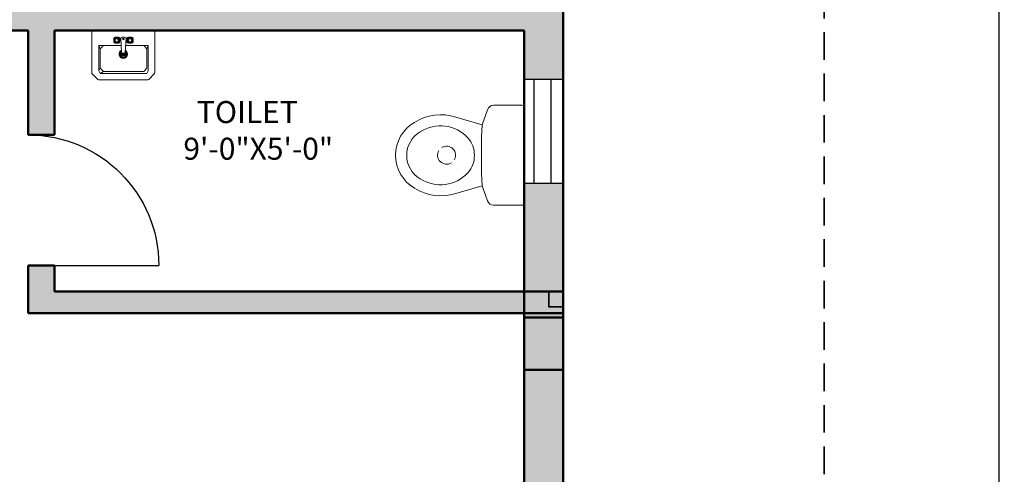
# Model space of a CAD drawing. Units: inches. Extents: x -7 to 1228, y -146 to 1091.
# Tile 41 of 88: x 1002 to 1228, y 200 to 304. Entities that reach past the tile are written whole.
import ezdxf

# ---------------------------------------------------------------- set-up
doc = ezdxf.new("R2010")
doc.units = ezdxf.units.IN
doc.linetypes.add('DASHED2', pattern=[9.525, 6.35, -3.175])
for name, color, linetype, lineweight in [('A-ANNO-DIMS', 2, 'Continuous', 18), ('A-AREA-IDEN', 7, 'Continuous', 18), ('A-COLS', 6, 'Continuous', 35), ('A-DOOR', 4, 'Continuous', 25), ('A-FLOR-FIXT', 8, 'Continuous', 18), ('A-FURN', 8, 'Continuous', 18), ('A-GLAZ', 175, 'Continuous', 25), ('A-WALL', 7, 'Continuous', 50), ('A-WALL-PATT', 251, 'Continuous', 13), ('C-PROP', 1, 'DASHED2', 35)]:
    doc.layers.add(name, color=color, linetype=linetype, lineweight=lineweight)
doc.styles.get("Standard").update_dxf_attribs({"font": 'arial.ttf'})
doc.dimstyles.new('ISO-25', dxfattribs={"dimtxt": 7, "dimasz": 4, "dimexe": 1.25, "dimexo": 0.625, "dimtad": 1, "dimdec": 1, "dimlunit": 3, "dimtxsty": 'Standard', "dimcen": 2.5, "dimadec": 0, "dimazin": 0, "dimtfac": 1, "dimtdec": 1, "dimtmove": 1, "dimatfit": 3, "dimfxl": 1, "dimarcsym": 0})

# ---------------------------------------------------------------- blocks, each defined once
blk = doc.blocks.new('A$C7B5C7CD4')
at = {"ltscale": 20}
for p, q in [((0.243, 0.625), (0.011, 0.625)), ((0.243, 0.625), (0.475, 0.625)), ((0, 0.614), (0, 0.4765)), ((0.486, 0.614), (0.486, 0.4765)), ((0.0212, 0.4467), (0.0946, 0.4214)), ((0.4648, 0.4467), (0.3914, 0.4214)), ((0.0946, 0.4214), (0.0576, 0.293)), ((0.0946, 0.4214), (0.1544, 0.4173)), ((0.3316, 0.4173), (0.1544, 0.4173)), ((0.3914, 0.4214), (0.3316, 0.4173)), ((0.3914, 0.4214), (0.4284, 0.293))]:
    blk.add_line(p, q, dxfattribs=at)
for centre, radius, start, end in [((0.011, 0.614), 0.011, 90, 180), ((0.475, 0.614), 0.011, 0, 90), ((0.0315, 0.4765), 0.0315, 180, 251), ((0.4545, 0.4765), 0.0315, 289, 0), ((0.2796, 0.219), 0.18, 132.4207, 213.289), ((0.24, 0.2602), 0.123, 88.6158, 131.7414), ((0.246, 0.2602), 0.123, 48.2586, 91.3842), ((0.2064, 0.219), 0.18, 326.711, 47.5793), ((0.2796, 0.219), 0.234, 161.5846, 212.8753), ((0.2064, 0.219), 0.234, 327.1247, 18.4154), ((0.243, 0.185), 0.131, 209.6292, 270), ((0.243, 0.185), 0.131, 270, 330.3708), ((0.243, 0.185), 0.185, 210.1745, 270), ((0.243, 0.185), 0.185, 270, 329.8255)]:
    blk.add_arc(centre, radius, start, end, dxfattribs=at)
for start, end in [(58.1785, 211.8215), (238.1785, 31.8215)]:
    blk.add_arc((0.2426, 0.2481), 0.0439, start, end)
blk = doc.blocks.new('*D12')
at = {"layer": 'A-ANNO-DIMS', "color": 0, "lineweight": -2, "transparency": 16777216}
for p, q in [((1187.62, 1061), (1228.45, 1061)), ((1227.2, 1057), (1227.2, 4)), ((1187.62, 0), (1228.45, 0))]:
    blk.add_line(p, q, dxfattribs=at)
at = {"layer": 'A-ANNO-DIMS', "color": 0, "transparency": 16777216}
for points in [[(1226.53, 1057), (1227.86, 1057), (1227.2, 1061)], [(1226.53, 4), (1227.86, 4), (1227.2, 0)]]:
    blk.add_solid(points, dxfattribs=at)
at = {"layer": 'Defpoints', "color": 0, "transparency": 16777216}
for p in [(1187, 1061), (1187, 0), (1227.2, 0)]:
    blk.add_point(p, dxfattribs=at)
at = {"layer": 'A-ANNO-DIMS', "color": 0, "transparency": 16777216, "insert": (1223, 530.5), "char_height": 7, "attachment_point": 5, "rotation": 90}
blk.add_mtext('88\'-5"', dxfattribs=at)
blk = doc.blocks.new('A$C4CB854FF')
for p, q in [((0.4725, 0.38), (0.0125, 0.38)), ((0, 0.3675), (0, 0.0552)), ((0.1677, 0.2932), (0.1677, 0.318)), ((0.1745, 0.2919), (0.1745, 0.3194)), ((0.1773, 0.3221), (0.2048, 0.3221)), ((0.1787, 0.329), (0.2034, 0.329)), ((0.2075, 0.3194), (0.2075, 0.2919)), ((0.2144, 0.318), (0.2144, 0.2932)), ((0.2279, 0.2104), (0.2213, 0.3235)), ((0.2337, 0.329), (0.2502, 0.329)), ((0.2625, 0.3235), (0.256, 0.2104)), ((0.2694, 0.318), (0.2694, 0.2932)), ((0.2763, 0.3194), (0.2763, 0.2919)), ((0.3065, 0.3221), (0.279, 0.3221)), ((0.3052, 0.329), (0.2804, 0.329)), ((0.3093, 0.2919), (0.3093, 0.3194)), ((0.3162, 0.2932), (0.3162, 0.318)), ((0.485, 0.0552), (0.485, 0.3675)), ((0.05, 0.265), (0.2247, 0.265)), ((0.06, 0.24), (0.05, 0.265)), ((0.05, 0.07), (0.05, 0.265)), ((0.085, 0.265), (0.06, 0.24)), ((0.06, 0.24), (0.06, 0.09)), ((0.2048, 0.2891), (0.1773, 0.2891)), ((0.2034, 0.2822), (0.1787, 0.2822)), ((0.2591, 0.265), (0.43, 0.265)), ((0.279, 0.2891), (0.3065, 0.2891)), ((0.2804, 0.2822), (0.3052, 0.2822)), ((0.395, 0.265), (0.42, 0.24)), ((0.42, 0.24), (0.43, 0.265)), ((0.42, 0.24), (0.42, 0.09)), ((0.43, 0.07), (0.43, 0.265)), ((0.2152, 0.1984), (0.2694, 0.1984)), ((0.2297, 0.2066), (0.2165, 0.2066)), ((0.2681, 0.1901), (0.2165, 0.1901)), ((0.2272, 0.2149), (0.2208, 0.2149)), ((0.2638, 0.1819), (0.2208, 0.1819)), ((0.2533, 0.1736), (0.2313, 0.1736)), ((0.2505, 0.2052), (0.2334, 0.2052)), ((0.2681, 0.2066), (0.2541, 0.2066)), ((0.2638, 0.2149), (0.2566, 0.2149)), ((0.06, 0.09), (0.085, 0.065)), ((0.42, 0.09), (0.395, 0.065)), ((0.42, 0.09), (0.43, 0.07)), ((0.0037, 0.0463), (0.0463, 0.0037)), ((0.05, 0.07), (0.06, 0.05)), ((0.42, 0.05), (0.06, 0.05)), ((0.085, 0.065), (0.395, 0.065)), ((0.395, 0.065), (0.42, 0.05)), ((0.43, 0.07), (0.42, 0.05)), ((0.4387, 0.0037), (0.4813, 0.0463)), ((0.0552, 0), (0.4298, 0))]:
    blk.add_line(p, q)
for centre, radius in [((0.191, 0.3056), 0.0165), ((0.191, 0.3056), 0.0127), ((0.2419, 0.3152), 0.00688), ((0.2419, 0.3152), 0.00344), ((0.2928, 0.3056), 0.0165), ((0.2928, 0.3056), 0.0127)]:
    blk.add_circle(centre, radius)
for centre, radius, start, end in [((0.0125, 0.3675), 0.0125, 90, 180), ((0.4725, 0.3675), 0.0125, 0, 90), ((0.1787, 0.318), 0.011, 90, 180), ((0.1773, 0.3194), 0.00275, 90, 180), ((0.2034, 0.318), 0.011, 0, 90), ((0.2048, 0.3194), 0.00275, 360, 90), ((0.2329, 0.314), 0.015, 87.19754, 140.72744), ((0.2509, 0.314), 0.015, 39.27256, 92.80246), ((0.2804, 0.318), 0.011, 90, 180), ((0.279, 0.3194), 0.00275, 90, 180), ((0.3052, 0.318), 0.011, 0, 90), ((0.3065, 0.3194), 0.00275, 360, 90), ((0.1787, 0.2932), 0.011, 180, 270), ((0.1773, 0.2919), 0.00275, 180, 270), ((0.2034, 0.2932), 0.011, 270, 0), ((0.2048, 0.2919), 0.00275, 270, 0), ((0.2423, 0.1984), 0.033, 118.68833, 62.86857), ((0.2804, 0.2932), 0.011, 180, 270), ((0.279, 0.2919), 0.00275, 180, 270), ((0.3052, 0.2932), 0.011, 270, 360), ((0.3065, 0.2919), 0.00275, 270, 0), ((0.2423, 0.1984), 0.0271, 124.77581, 57.22467), ((0.2334, 0.2107), 0.0055, 183.3274, 270), ((0.2505, 0.2107), 0.0055, 270, 356.6726), ((0.0125, 0.0552), 0.0125, 180, 225), ((0.0552, 0.0125), 0.0125, 225, 270), ((0.4298, 0.0125), 0.0125, 270, 315), ((0.4725, 0.0552), 0.0125, 315, 0)]:
    blk.add_arc(centre, radius, start, end)
blk = doc.blocks.new('WIN-24')
for p, q in [((0, 0), (0, 24)), ((0, 24), (9, 24)), ((2.34, 0), (2.34, 24)), ((2.34, 24), (6.14, 24)), ((6.14, 24), (6.14, 0)), ((9, 24), (9, 0)), ((9, 0), (0, 0))]:
    blk.add_line(p, q)
blk = doc.blocks.new('DOOR-750')
blk.add_line((30, 30), (30, 0))
blk.add_arc((30, 30), 30, 180, 270)

msp = doc.modelspace()

# ---------------------------------------------------------------- hatches: boundary and pattern name
at = {"layer": 'A-COLS'}
h = msp.add_hatch(color=256, dxfattribs=at)
h.dxf.hatch_style = 1
h.paths.add_polyline_path([(1127, 238.45), (1123.71, 238.45), (1123.71, 242), (1118, 242), (1118, 224), (1127, 224)])
h = msp.add_hatch(color=256, dxfattribs=at)
h.dxf.hatch_style = 1
h.paths.add_polyline_path([(1127, 238.45), (1127, 242), (1123.71, 242), (1123.71, 238.45)])
at = {"layer": 'A-WALL-PATT'}
h = msp.add_hatch(color=256, dxfattribs=at)
h.dxf.hatch_style = 1
h.paths.add_polyline_path([(69, 568), (60, 568), (60, 493), (63.29, 493), (69, 493)])
h.paths.add_polyline_path([(69, 662.41), (60, 662.41), (60, 586), (69, 586)], flags=17)
h.paths.add_polyline_path([(69, 723), (184, 723), (184, 734), (179, 734), (179, 728), (69, 728), (69, 741.62), (60, 741.62), (60, 698.41), (69, 698.41)], flags=17)
h.paths.add_polyline_path([(69, 782), (231, 782), (231, 728), (231, 723), (231, 586), (236, 586), (236, 787), (69, 787), (69, 800.13), (60, 800.13), (60, 765.62), (69, 765.62)])
h.paths.add_polyline_path([(184, 842), (189, 842), (189, 848), (173, 848), (173, 842), (179, 842), (179, 787), (184, 787)])
h.paths.add_polyline_path([(118.22, 69), (69, 69), (69, 60), (118.22, 60)])
h.paths.add_polyline_path([(227, 69), (154.22, 69), (154.22, 60), (227, 60)])
h.paths.add_polyline_path([(236, 60), (232.71, 60), (227, 60), (227, 36), (236, 36)])
h.paths.add_polyline_path([(389, 60), (380, 60), (380, 36), (389, 36)])
h.paths.add_polyline_path([(384, 181), (380, 181), (380, 115), (380, 78), (384, 78)])
h.paths.add_polyline_path([(380, 115), (334.55, 115), (334.55, 109), (380, 109)])
h.paths.add_polyline_path([(274.55, 115), (236, 115), (236, 201), (232.71, 201), (231, 201), (231, 78), (236, 78), (236, 109), (274.55, 109)])
h.paths.add_polyline_path([(69, 123), (60, 123), (60, 78), (69, 78)])
h.paths.add_polyline_path([(69, 201), (60, 201), (60, 159), (69, 159)])
h.paths.add_polyline_path([(143, 219), (69, 219), (69, 213), (143, 213)], flags=17)
h.paths.add_polyline_path([(189, 219), (184, 219), (184, 274), (231, 274), (231, 219), (236, 219), (236, 279), (184, 279), (184, 297), (179, 297), (179, 279), (69, 279), (69, 290.91), (60, 290.91), (60, 262.18), (69, 262.18), (69, 274), (179, 274), (179, 219), (173, 219), (173, 213), (189, 213)])
h.paths.add_polyline_path([(69, 238.18), (60, 238.18), (60, 219), (69, 219)], flags=17)
h.paths.add_polyline_path([(69, 333), (60, 333), (60, 314.91), (69, 314.91), (69, 316.96)])
h.paths.add_polyline_path([(190, 338), (184, 338), (69, 338), (69, 333), (179, 333), (179, 327), (184, 327), (184, 333.02), (190, 333.05)])
h.paths.add_polyline_path([(69, 386.81), (60, 386.81), (60, 351), (69, 351)])
h.paths.add_polyline_path([(69, 475), (60, 475), (60, 422.81), (69, 422.81)])
h.paths.add_polyline_path([(236, 475), (231, 475), (231, 351.24), (236, 351.24)])
h.paths.add_polyline_path([(384, 475), (380, 475), (380, 362), (384, 362)])
h.paths.add_polyline_path([(547, 307), (439, 307), (439, 356), (445, 356), (445, 362), (433, 362), (433, 307), (380, 307), (380, 244), (380, 241), (384, 241), (384, 301), (433, 301), (433, 277), (439, 277), (439, 301), (547, 301)])
h.paths.add_polyline_path([(547, 241), (439, 241), (439, 247), (433, 247), (433, 235), (547, 235)])
h.paths.add_polyline_path([(450, 69), (440.29, 69), (424.89, 69), (389, 69), (389, 60), (450, 60)])
h.paths.add_polyline_path([(547, 69), (486, 69), (486, 60), (547, 60)])
h.paths.add_polyline_path([(556, 148.27), (547, 148.27), (547, 78), (556, 78)])
h.paths.add_polyline_path([(556, 223), (547, 223), (547, 195), (547, 184.27), (556, 184.27)])
h.paths.add_polyline_path([(556, 311.19), (547, 311.19), (547, 273.08), (556, 273.08)])
h.paths.add_polyline_path([(556, 344), (552.71, 344), (547, 344), (547, 335.19), (556, 335.19)])
h.paths.add_polyline_path([(556, 249.08), (547, 249.08), (547, 241), (556, 241)])
h.paths.add_polyline_path([(547, 362), (475, 362), (475, 356), (547, 356)], flags=0)
h.paths.add_polyline_path([(556, 399.62), (547, 399.62), (547, 362), (556, 362)])
h.paths.add_polyline_path([(556, 475), (547, 475), (547, 435.62), (556, 435.62)])
h.paths.add_polyline_path([(547, 493), (389, 493), (389, 487), (547, 487)])
h.paths.add_polyline_path([(380, 493), (278, 493), (278, 487), (380, 487)])
h.paths.add_polyline_path([(227, 493), (69, 493), (69, 487), (227, 487)])
h.paths.add_polyline_path([(643, 122.44), (634, 122.44), (634, 78), (643, 78)])
h.paths.add_polyline_path([(702.5, 69), (692.79, 69), (677.39, 69), (643, 69), (643, 60), (702.5, 60)])
h.paths.add_polyline_path([(798, 69), (738.5, 69), (738.5, 60), (798, 60)])
h.paths.add_polyline_path([(807, 60), (803.71, 60), (798, 60), (798, 36), (807, 36)])
h.paths.add_polyline_path([(807, 109), (846.75, 109), (846.75, 115), (807, 115), (807, 159), (802, 159), (802, 78), (807, 78)])
h.paths.add_polyline_path([(807, 201), (802, 201), (802, 195), (807, 195)])
h.paths.add_polyline_path([(643, 201), (634, 201), (634, 158.44), (643, 158.44)])
h.paths.add_polyline_path([(756, 225), (751, 225), (751, 219), (643, 219), (643, 213), (756, 213)])
h.paths.add_polyline_path([(643, 240.85), (634, 240.85), (634, 219), (643, 219)])
h.paths.add_polyline_path([(643, 274), (643, 288.63), (634, 288.63), (634, 264.85), (643, 264.85)])
h.paths.add_polyline_path([(802, 279), (756, 279), (756, 297), (751, 297), (751, 279), (643, 279), (643, 274), (751, 274), (751, 255), (756, 255), (756, 274), (802, 274)])
h.paths.add_polyline_path([(807, 333), (803.71, 333), (802, 333), (802, 279), (802, 274), (802, 219), (807, 219)])
h.paths.add_polyline_path([(956, 182), (951, 182), (951, 115), (906.75, 115), (906.75, 109), (951, 109), (951, 78), (956, 78)])
h.paths.add_polyline_path([(960, 60), (951, 60), (951, 36), (960, 36)])
h.paths.add_polyline_path([(1021, 69), (1005.78, 69), (960, 69), (960, 60), (1021, 60)])
h.paths.add_polyline_path([(956, 224), (951, 224), (951, 218), (956, 218)])
h.paths.add_polyline_path([(956, 302), (1004, 302), (1004, 278), (1010, 278), (1010, 302), (1118, 302), (1118, 290.81), (1127, 290.81), (1127, 326.97), (1118, 326.97), (1118, 320.97), (1118, 307), (1010, 307), (1010, 356), (1016, 356), (1016, 362), (1004, 362), (1004, 307), (951, 307), (951, 244), (951, 242), (954.29, 242), (956, 242)])
h.paths.add_polyline_path([(643, 333), (634, 333), (634, 312.63), (643, 312.63), (643, 316.96)])
h.paths.add_polyline_path([(756, 338), (643, 338), (643, 333), (751, 333), (751, 327), (756, 327)])
h.paths.add_polyline_path([(643, 388), (634, 388), (634, 351), (643, 351)])
h.paths.add_polyline_path([(807, 357), (802, 357), (802, 351), (807, 351)])
h.paths.add_polyline_path([(807, 475), (802, 475), (802, 393), (807, 393)])
h.paths.add_polyline_path([(643, 475), (634, 475), (634, 424), (643, 424)])
h.paths.add_polyline_path([(798, 493), (643, 493), (643, 487), (798, 487)])
h.paths.add_polyline_path([(634, 493), (556, 493), (556, 487), (634, 487)])
h.paths.add_polyline_path([(813, 493), (807, 493), (807, 487), (813, 487)])
h.paths.add_polyline_path([(951, 493), (849, 493), (849, 487), (951, 487)])
h.paths.add_polyline_path([(956, 484), (951, 484), (951, 374), (956, 374)])
h.paths.add_polyline_path([(1109, 493), (969, 493), (969, 487), (1109, 487)])
h.paths.add_polyline_path([(1127, 484), (1118, 484), (1118, 450.64), (1127, 450.64)])
h.paths.add_polyline_path([(1127, 414.64), (1118, 414.64), (1118, 365), (1127, 365)])
h.paths.add_polyline_path([(1109, 362), (1046, 362), (1046, 356), (1109, 356)], flags=17)
h.paths.add_polyline_path([(1127, 356), (1123.45, 356), (1118, 356), (1118, 350.97), (1127, 350.97)], flags=0)
h.paths.add_polyline_path([(1127, 266.81), (1118, 266.81), (1118, 262.36), (1118, 242), (1127, 242)], flags=17)
h.paths.add_polyline_path([(1118, 242), (1010, 242), (1010, 248), (1004, 248), (1004, 237), (1118, 237)])
h.paths.add_polyline_path([(1127, 224), (1118, 224), (1118, 170), (1127, 170)])
h.paths.add_polyline_path([(1127, 134), (1118, 134), (1118, 78), (1127, 78)])
h.paths.add_polyline_path([(1118, 69), (1057, 69), (1057, 60), (1118, 60)])
h.paths.add_polyline_path([(227, 571.55), (227, 574), (69, 574), (69, 568), (227, 568)])
h.paths.add_polyline_path([(380, 571.55), (380, 574), (278, 574), (278, 568), (380, 568)])
h.paths.add_polyline_path([(242, 574), (236, 574), (236, 568), (242, 568)])
h.paths.add_polyline_path([(547, 571.55), (547, 574), (389, 574), (389, 568), (547, 568)])
h.paths.add_polyline_path([(384, 733), (380, 733), (380, 586), (384, 586)])
h.paths.add_polyline_path([(556, 646), (634, 646), (634, 655), (547, 655), (547, 586), (556, 586)])
h.paths.add_polyline_path([(634, 574), (556, 574), (556, 568), (634, 568)])
h.paths.add_polyline_path([(643, 655), (634, 655), (634, 586), (643, 586)])
h.paths.add_polyline_path([(798, 574), (643, 574), (643, 568), (798, 568)])
h.paths.add_polyline_path([(643, 663.85), (634, 663.85), (634, 655), (643, 655)])
h.paths.add_polyline_path([(556, 676.97), (547, 676.97), (547, 655), (556, 655)])
h.paths.add_polyline_path([(556, 733), (547, 733), (547, 712.97), (556, 712.97)])
h.paths.add_polyline_path([(643, 710), (634, 710), (634, 699.85), (643, 699.85)])
h.paths.add_polyline_path([(807, 668), (802, 668), (802, 586), (807, 586)])
h.paths.add_polyline_path([(951, 574), (849, 574), (849, 568), (951, 568)])
h.paths.add_polyline_path([(956, 691), (951, 691), (951, 577), (956, 577)])
h.paths.add_polyline_path([(1109, 574), (969, 574), (969, 568), (1109, 568)])
h.paths.add_polyline_path([(1127, 643.4), (1118, 643.4), (1118, 577), (1127, 577)])
h.paths.add_polyline_path([(1127, 568), (1123.45, 568), (1118, 568), (1118, 493), (1127, 493)])
h.paths.add_polyline_path([(1127, 733), (1118, 733), (1118, 679.4), (1127, 679.4)])
h.paths.add_polyline_path([(1127, 777.35), (1118, 777.35), (1118, 770.04), (1118, 751), (1127, 751)], flags=17)
h.paths.add_polyline_path([(1118, 751), (1010, 751), (1010, 757), (1004, 757), (1004, 745), (1118, 745)])
h.paths.add_polyline_path([(956, 811), (1004, 811), (1004, 787), (1010, 787), (1010, 811), (1017.87, 811), (1017.87, 811.63, -0.414214), (1018.25, 812), (1031.98, 812, -0.414214), (1032.35, 811.63), (1032.35, 811), (1118, 811), (1118, 801.35), (1127, 801.35), (1127, 834.69), (1118, 834.69), (1118, 830.24), (1118, 817), (1010, 817), (1010, 866), (1016, 866), (1016, 872), (1004, 872), (1004, 817), (956, 817), (956, 866), (951, 866), (951, 751), (954.29, 751), (956, 751)])
h.paths.add_polyline_path([(1118, 872), (1046, 872), (1046, 866), (1118, 866)], flags=17)
h.paths.add_polyline_path([(1127, 924.71), (1118, 924.71), (1118, 884), (1127, 884)])
h.paths.add_polyline_path([(1127, 866), (1123.71, 866), (1118, 866), (1118, 858.69), (1127, 858.69)], flags=17)
h.paths.add_polyline_path([(956, 983), (951, 983), (951, 952), (807, 952), (807, 983), (802, 983), (802, 902), (807, 902), (807, 946), (951, 946), (951, 884), (956, 884)])
h.paths.add_polyline_path([(807, 842), (802, 842), (802, 787), (756, 787), (756, 806), (751, 806), (751, 787), (643, 787), (643, 782), (751, 782), (751, 764), (756, 764), (756, 782), (802, 782), (802, 728), (807, 728)])
h.paths.add_polyline_path([(756, 848), (643, 848), (643, 842), (751, 842), (751, 836), (756, 836)])
h.paths.add_polyline_path([(756, 734), (751, 734), (751, 728), (643, 728), (643, 723), (756, 723)])
h.paths.add_polyline_path([(643, 749.79), (634, 749.79), (634, 728), (637.29, 728), (643, 728)])
h.paths.add_polyline_path([(643, 805.41), (634, 805.41), (634, 773.79), (643, 773.79)])
h.paths.add_polyline_path([(643, 896.66), (634, 896.66), (634, 860), (637.29, 860), (643, 860)])
h.paths.add_polyline_path([(643, 842), (634, 842), (634, 829.41), (643, 829.41)])
h.paths.add_polyline_path([(643, 983), (634, 983), (634, 932.66), (643, 932.66)])
h.paths.add_polyline_path([(1127, 983), (1118, 983), (1118, 960.71), (1127, 960.71)])
h.paths.add_polyline_path([(1118, 1001), (1077.53, 1001), (1077.53, 992), (1118, 992)])
h.paths.add_polyline_path([(1041.53, 1001), (960, 1001), (960, 992), (1041.53, 992)])
h.paths.add_polyline_path([(960, 1025), (951, 1025), (951, 1001), (954.29, 1001), (960, 1001)])
h.paths.add_polyline_path([(807, 1025), (798, 1025), (798, 1001), (807, 1001)])
h.paths.add_polyline_path([(798, 1001), (738.5, 1001), (738.5, 992), (798, 992)])
h.paths.add_polyline_path([(702.5, 1001), (643, 1001), (643, 992), (702.5, 992)])
h.paths.add_polyline_path([(547, 1001), (499.11, 1001), (499.11, 992), (547, 992)])
h.paths.add_polyline_path([(463.11, 1001), (389, 1001), (389, 992), (463.11, 992)])
h.paths.add_polyline_path([(389, 1025), (380, 1025), (380, 1022), (380, 1001), (383.29, 1001), (389, 1001)])
h.paths.add_polyline_path([(236, 1025), (227, 1025), (227, 1001), (236, 1001)])
h.paths.add_polyline_path([(236, 983), (231, 983), (231, 860), (236, 860)])
h.paths.add_polyline_path([(274.55, 952), (236, 952), (236, 946), (274.55, 946)])
h.paths.add_polyline_path([(380, 952), (334.55, 952), (334.55, 946), (380, 946)])
h.paths.add_polyline_path([(384, 983), (380, 983), (380, 884), (383.29, 884), (384, 884)])
h.paths.add_polyline_path([(227, 1001), (155.01, 1001), (155.01, 992), (162.87, 992), (227, 992)])
h.paths.add_polyline_path([(119.01, 1001), (69, 1001), (69, 992), (119.01, 992)])
h.paths.add_polyline_path([(69, 983), (60, 983), (60, 922.99), (69, 922.99)])
h.paths.add_polyline_path([(69, 886.99), (60, 886.99), (60, 860), (63.29, 860), (69, 860)])
h.paths.add_polyline_path([(143, 848), (69, 848), (69, 842), (143, 842)])

# ---------------------------------------------------------------- linework, layer by layer
at = {"layer": 'A-COLS'}
msp.add_lwpolyline([(1127, 242), (1123.71, 242), (1123.71, 238.45), (1127, 238.45)], close=True, dxfattribs=at)
at = {"layer": 'A-WALL'}
for p, q in [((1127, 60), (1127, 1001)), ((1004, 302), (956, 302)), ((1004, 278), (1004, 302)), ((1118, 302), (1010, 302)), ((1010, 278), (1010, 302)), ((1118, 60), (1118, 302)), ((1010, 278), (1004, 278)), ((1004, 237), (1004, 248)), ((1010, 248), (1004, 248)), ((1010, 242), (1010, 248)), ((1118, 244), (1118, 60)), ((1127, 242), (1010, 242)), ((1127, 242), (1118, 242)), ((1127, 242), (1118, 242)), ((1118, 242), (1118, 224)), ((1127, 224), (1127, 242)), ((1127, 237), (1004, 237)), ((1127, 236), (1118, 236)), ((1118, 224), (1127, 224))]:
    msp.add_line(p, q, dxfattribs=at)
at = {"layer": 'C-PROP'}
msp.add_line((1187, 0), (1187, 1061), dxfattribs=at)

# ---------------------------------------------------------------- block references
at = {"layer": 'A-DOOR', "extrusion": (0, 0, -1), "zscale": -1, "rotation": 270.0000000000009}
msp.add_blockref('DOOR-750', (-1034, 278), dxfattribs=at)
at = {"layer": 'A-FLOR-FIXT', "xscale": 47.26153857112405, "yscale": 47.26153857112405, "zscale": 47.26153857112405, "rotation": 270}
msp.add_blockref('A$C7B5C7CD4', (1088.46, 284.81), dxfattribs=at)
at = {"layer": 'A-FURN', "xscale": -29.84864686937646, "yscale": 29.84864686937646, "zscale": 29.84864686937646}
msp.add_blockref('A$C4CB854FF', (1033.08, 290.66), dxfattribs=at)
at = {"layer": 'A-GLAZ'}
msp.add_blockref('WIN-24', (1118, 266.81), dxfattribs=at)

# ---------------------------------------------------------------- texts
at = {"layer": 'A-AREA-IDEN', "insert": (1039.66, 285.79), "char_height": 5.0568, "attachment_point": 1}
msp.add_mtext_dynamic_manual_height_columns('  TOILET\\P9\'-0"X5\'-0"', width=137.2821, gutter_width=25.28, heights=[0], dxfattribs=at)

# ---------------------------------------------------------------- dimensions: what is measured, and where the dimension line sits
at = {"layer": 'A-ANNO-DIMS'}
dim = msp.add_linear_dim(base=(1227.2, 0), p1=(1187, 1061), p2=(1187, 0), angle=90, dimstyle='ISO-25', override={"dimclrd": 0, "dimclre": 0, "dimclrt": 0}, dxfattribs=at)
dim.commit()
dim.dimension.update_dxf_attribs({"geometry": '*D12', "text_midpoint": (1223, 530.5)})

doc.saveas('drawing.dxf')
